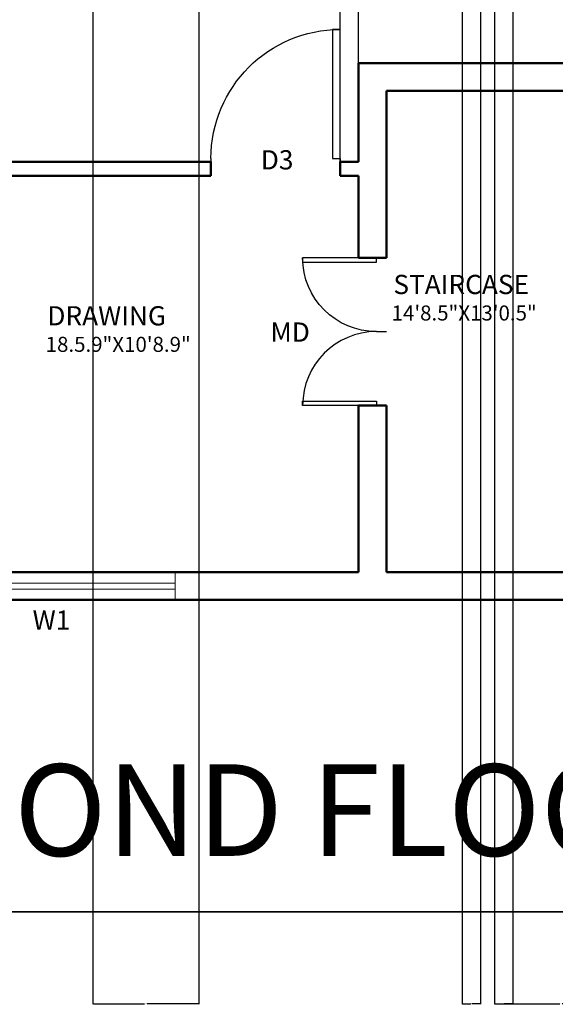
# Model space of a CAD drawing. Units: inches. Extents: x 7359 to 7979, y 33027 to 34263.
# Tile 4 of 32: x 7589 to 7764, y 33027 to 33347. Entities that reach past the tile are written whole.
import ezdxf

# ---------------------------------------------------------------- set-up
doc = ezdxf.new("R2010")
doc.units = ezdxf.units.IN
for name, color, linetype, lineweight in [('A-ANNO-DIMS', 2, 'Continuous', 18), ('A-ANNO-TEXT', 3, 'Continuous', 18), ('A-ANNO-TITL', 7, 'Continuous', 35), ('A-AREA-IDEN', 7, 'Continuous', 18), ('A-DOOR', 3, 'Continuous', 25), ('A-GLAZ', 4, 'Continuous', 18), ('A-WALL', 7, 'Continuous', 50)]:
    doc.layers.add(name, color=color, linetype=linetype, lineweight=lineweight)
doc.styles.get("Standard").update_dxf_attribs({"font": 'arial.ttf'})
doc.dimstyles.get("Standard").update_dxf_attribs({"dimtxt": 0.18, "dimasz": 0.18, "dimexe": 0.18, "dimexo": 0.0625, "dimgap": 0.09, "dimtad": 0, "dimtih": 1, "dimtoh": 1, "dimdec": 4, "dimzin": 0, "dimdsep": 46, "dimtxsty": 'Standard', "dimcen": 0.09, "dimadec": 0, "dimazin": 0, "dimtfac": 1, "dimtdec": 4, "dimtofl": 0, "dimtmove": 0, "dimatfit": 3, "dimfxl": 1, "dimtolj": 1, "dimtzin": 0, "dimarcsym": 0})

# ---------------------------------------------------------------- blocks, each defined once
blk = doc.blocks.new('*U2')
for p, q in [((0, 0), (0, -100)), ((750, 0), (750, -100))]:
    blk.add_line(p, q)
blk.add_lwpolyline([(0, 0), (0, 750), (43.75, 750), (43.75, 0)], close=True)
blk.add_arc((0, 0), 750, 0, 90)
blk = doc.blocks.new('WINDOW-W1-DRAWING-FRONT')
for p, q in [((0, 0), (0, 9)), ((78.79, 0), (78.79, 9)), ((0, 5.5), (78.79, 5.5)), ((0, 3.5), (78.79, 3.5))]:
    blk.add_line(p, q)
blk = doc.blocks.new('*D73')
at = {"layer": 'A-ANNO-DIMS', "color": 0, "lineweight": -2, "transparency": 16777216}
for p, q in [((7613.23, 33618.1), (7613.23, 33027.18)), ((7647.71, 33618.1), (7647.71, 33027.18)), ((7613.41, 33027.36), (7630.07, 33027.36)), ((7647.53, 33027.36), (7630.86, 33027.36))]:
    blk.add_line(p, q, dxfattribs=at)
at = {"layer": 'A-ANNO-DIMS', "color": 0, "transparency": 16777216}
for points in [[(7613.41, 33027.39), (7613.41, 33027.33), (7613.23, 33027.36)], [(7647.53, 33027.39), (7647.53, 33027.33), (7647.71, 33027.36)]]:
    blk.add_solid(points, dxfattribs=at)
at = {"layer": 'Defpoints', "color": 0, "transparency": 16777216}
for p in [(7613.23, 33618.16), (7647.71, 33618.16), (7647.71, 33027.36)]:
    blk.add_point(p, dxfattribs=at)
at = {"layer": 'A-ANNO-DIMS', "color": 0, "transparency": 16777216, "insert": (7630.47, 33027.36), "char_height": 0.18, "attachment_point": 5}
blk.add_mtext('\\A1;34.48', dxfattribs=at)
blk = doc.blocks.new('*D74')
at = {"layer": 'A-ANNO-DIMS', "color": 0, "lineweight": -2, "transparency": 16777216}
for p, q in [((7743.73, 33618.1), (7743.73, 33027.18)), ((7787.03, 33618.1), (7787.03, 33027.18)), ((7743.91, 33027.36), (7765, 33027.36)), ((7786.85, 33027.36), (7765.76, 33027.36))]:
    blk.add_line(p, q, dxfattribs=at)
at = {"layer": 'A-ANNO-DIMS', "color": 0, "transparency": 16777216}
for points in [[(7743.91, 33027.39), (7743.91, 33027.33), (7743.73, 33027.36)], [(7786.85, 33027.39), (7786.85, 33027.33), (7787.03, 33027.36)]]:
    blk.add_solid(points, dxfattribs=at)
at = {"layer": 'Defpoints', "color": 0, "transparency": 16777216}
for p in [(7743.73, 33618.16), (7787.03, 33618.16), (7787.03, 33027.36)]:
    blk.add_point(p, dxfattribs=at)
at = {"layer": 'A-ANNO-DIMS', "color": 0, "transparency": 16777216, "insert": (7765.38, 33027.36), "char_height": 0.18, "attachment_point": 5}
blk.add_mtext('\\A1;43.31', dxfattribs=at)
blk = doc.blocks.new('*D86')
at = {"layer": 'A-ANNO-DIMS', "color": 0, "lineweight": -2, "transparency": 16777216}
for p, q in [((7733.226578, 33475.599789), (7733.226578, 33027.176807)), ((7739.226578, 33475.599789), (7739.226578, 33027.176807)), ((7733.406578, 33027.356807), (7736.077151, 33027.356807)), ((7739.046578, 33027.356807), (7736.376005, 33027.356807))]:
    blk.add_line(p, q, dxfattribs=at)
at = {"layer": 'A-ANNO-DIMS', "color": 0, "transparency": 16777216}
for points in [[(7733.406578, 33027.386807), (7733.406578, 33027.326807), (7733.226578, 33027.356807)], [(7739.046578, 33027.386807), (7739.046578, 33027.326807), (7739.226578, 33027.356807)]]:
    blk.add_solid(points, dxfattribs=at)
at = {"layer": 'Defpoints', "color": 0, "transparency": 16777216}
for p in [(7733.226578, 33475.662289), (7739.226578, 33475.662289), (7739.226578, 33027.356807)]:
    blk.add_point(p, dxfattribs=at)
at = {"layer": 'A-ANNO-DIMS', "color": 0, "transparency": 16777216, "insert": (7736.226578, 33027.356807), "char_height": 0.18, "attachment_point": 5}
blk.add_mtext('\\A1;6', dxfattribs=at)
blk = doc.blocks.new('*D87')
at = {"layer": 'A-ANNO-DIMS', "color": 0, "lineweight": -2, "transparency": 16777216}
for p, q in [((7743.726578, 33453.099789), (7743.726578, 33027.176807)), ((7749.726578, 33453.099789), (7749.726578, 33027.176807)), ((7743.906578, 33027.356807), (7746.577151, 33027.356807)), ((7749.546578, 33027.356807), (7746.876005, 33027.356807))]:
    blk.add_line(p, q, dxfattribs=at)
at = {"layer": 'A-ANNO-DIMS', "color": 0, "transparency": 16777216}
for points in [[(7743.906578, 33027.386807), (7743.906578, 33027.326807), (7743.726578, 33027.356807)], [(7749.546578, 33027.386807), (7749.546578, 33027.326807), (7749.726578, 33027.356807)]]:
    blk.add_solid(points, dxfattribs=at)
at = {"layer": 'Defpoints', "color": 0, "transparency": 16777216}
for p in [(7743.726578, 33453.162289), (7749.726578, 33453.162289), (7749.726578, 33027.356807)]:
    blk.add_point(p, dxfattribs=at)
at = {"layer": 'A-ANNO-DIMS', "color": 0, "transparency": 16777216, "insert": (7746.726578, 33027.356807), "char_height": 0.18, "attachment_point": 5}
blk.add_mtext('\\A1;6', dxfattribs=at)
blk = doc.blocks.new('*D89')
at = {"layer": 'A-ANNO-DIMS', "color": 0, "lineweight": -2, "transparency": 16777216}
for p, q in [((7693.626578, 33301.124789), (7693.626578, 33657.242289)), ((7693.806578, 33657.062289), (7696.477151, 33657.062289)), ((7699.446578, 33657.062289), (7696.776005, 33657.062289)), ((7699.626578, 33301.124789), (7699.626578, 33657.242289))]:
    blk.add_line(p, q, dxfattribs=at)
at = {"layer": 'A-ANNO-DIMS', "color": 0, "transparency": 16777216}
for points in [[(7693.806578, 33657.092289), (7693.806578, 33657.032289), (7693.626578, 33657.062289)], [(7699.446578, 33657.092289), (7699.446578, 33657.032289), (7699.626578, 33657.062289)]]:
    blk.add_solid(points, dxfattribs=at)
at = {"layer": 'Defpoints', "color": 0, "transparency": 16777216}
for p in [(7699.626578, 33657.062289), (7693.626578, 33301.062289), (7699.626578, 33301.062289)]:
    blk.add_point(p, dxfattribs=at)
at = {"layer": 'A-ANNO-DIMS', "color": 0, "transparency": 16777216, "insert": (7696.626578, 33657.062289), "char_height": 0.18, "attachment_point": 5}
blk.add_mtext('\\A1;6', dxfattribs=at)

msp = doc.modelspace()

# ---------------------------------------------------------------- linework, layer by layer
at = {"layer": 'A-ANNO-TITL'}
msp.add_line((7520.8378, 33057.2568), (7859.2391, 33057.2568), dxfattribs=at)
at = {"layer": 'A-WALL'}
for p, q in [((7699.6266, 33333.1623), (7788.6266, 33333.1623)), ((7699.6266, 33333.1623), (7699.6266, 33301.0623)), ((7708.6266, 33324.1623), (7885.1266, 33324.1623)), ((7708.6266, 33324.1623), (7708.6266, 33269.9123)), ((7477.7266, 33301.0623), (7651.6266, 33301.0623)), ((7651.6266, 33301.0623), (7651.6266, 33296.5623)), ((7693.6266, 33301.0623), (7699.6266, 33301.0623)), ((7693.6266, 33301.0623), (7693.6266, 33296.5623)), ((7477.7266, 33296.5623), (7651.6266, 33296.5623)), ((7693.6266, 33296.5623), (7699.6266, 33296.5623)), ((7699.6266, 33296.5623), (7699.6266, 33269.9123)), ((7708.6266, 33269.9123), (7699.6266, 33269.9123)), ((7699.6266, 33221.9123), (7699.6266, 33167.6623)), ((7708.6266, 33221.9123), (7699.6266, 33221.9123)), ((7708.6266, 33221.9123), (7708.6266, 33167.6623)), ((7477.7266, 33167.6623), (7699.6266, 33167.6623)), ((7708.6266, 33167.6623), (7885.1266, 33167.6623)), ((7468.7266, 33158.6623), (7894.1266, 33158.6623))]:
    msp.add_line(p, q, dxfattribs=at)

# ---------------------------------------------------------------- block references
at = {"layer": 'A-DOOR', "xscale": -0.0559999819687567, "yscale": 0.0559999819687567, "zscale": 0.0559999819687567}
msp.add_blockref('*U2', (7693.6266, 33302.1623), dxfattribs=at)
at = {"layer": 'A-DOOR', "yscale": 0.0319999999999999, "zscale": 0.0319999999999999, "rotation": 90}
for p, xscale in [((7705.4266, 33269.9123), -0.0319999999999999), ((7705.4266, 33221.9123), 0.0319999999999999)]:
    msp.add_blockref('*U2', p, dxfattribs=dict(at, xscale=xscale))
at = {"layer": 'A-GLAZ', "rotation": 180}
msp.add_blockref('WINDOW-W1-DRAWING-FRONT', (7640.013, 33167.6622), dxfattribs=at)

# ---------------------------------------------------------------- texts
at = {"layer": 'A-ANNO-TEXT'}
for s, p in [('D3', (7667.823, 33298.6351)), ('MD', (7670.9595, 33242.6245)), ('W1', (7593.6772, 33148.9717))]:
    msp.add_text(s, height=6.25941, dxfattribs=at).set_placement(p)
at = {"layer": 'A-ANNO-TITL'}
msp.add_text('SECOND FLOOR', height=29.769676, dxfattribs=at).set_placement((7513.5868, 33075.4364))
at = {"layer": 'A-AREA-IDEN'}
for s, height, p in [('STAIRCASE', 6.25941, (7710.905, 33258.1098)), ('14\'8.5"X13\'0.5"', 4.885549, (7710.3418, 33249.5154)), ('DRAWING', 6.25941, (7598.4692, 33247.9187)), ('18.5.9"X10\'8.9"', 4.885549, (7597.906, 33239.3243))]:
    msp.add_text(s, height=height, dxfattribs=at).set_placement(p)

# ---------------------------------------------------------------- dimensions: what is measured, and where the dimension line sits
at = {"layer": 'A-ANNO-DIMS'}
for base, p1, p2, override, picture, middle in [((7699.6266, 33657.0623), (7693.6266, 33301.0623), (7699.6266, 33301.0623), {"dimdec": 0, "dimlfac": 1, "dimrnd": 0, "dimzin": 0, "dimdsep": 46, "dimlunit": 2}, '*D89', (7696.6266, 33657.0623)), ((7647.7062, 33027.3568), (7613.2266, 33618.1623), (7647.7062, 33618.1623), {"dimdec": 2, "dimlfac": 1, "dimrnd": 0, "dimzin": 0, "dimdsep": 46, "dimlunit": 2}, '*D73', (7630.4664, 33027.3568)), ((7787.0342, 33027.3568), (7743.7266, 33618.1623), (7787.0342, 33618.1623), {"dimdec": 2, "dimlfac": 1, "dimrnd": 0, "dimzin": 0, "dimdsep": 46, "dimlunit": 2}, '*D74', (7765.3804, 33027.3568)), ((7739.2266, 33027.3568), (7733.2266, 33475.6623), (7739.2266, 33475.6623), {"dimdec": 0, "dimlfac": 1, "dimrnd": 0, "dimzin": 0, "dimdsep": 46, "dimlunit": 2}, '*D86', (7736.2266, 33027.3568)), ((7749.7266, 33027.3568), (7743.7266, 33453.1623), (7749.7266, 33453.1623), {"dimdec": 0, "dimlfac": 1, "dimrnd": 0, "dimzin": 0, "dimdsep": 46, "dimlunit": 2}, '*D87', (7746.7266, 33027.3568))]:
    dim = msp.add_linear_dim(base=base, p1=p1, p2=p2, dimstyle='Standard', override=override, dxfattribs=at)
    dim.commit()
    dim.dimension.update_dxf_attribs({"geometry": picture, "text_midpoint": middle})

doc.saveas('drawing.dxf')
